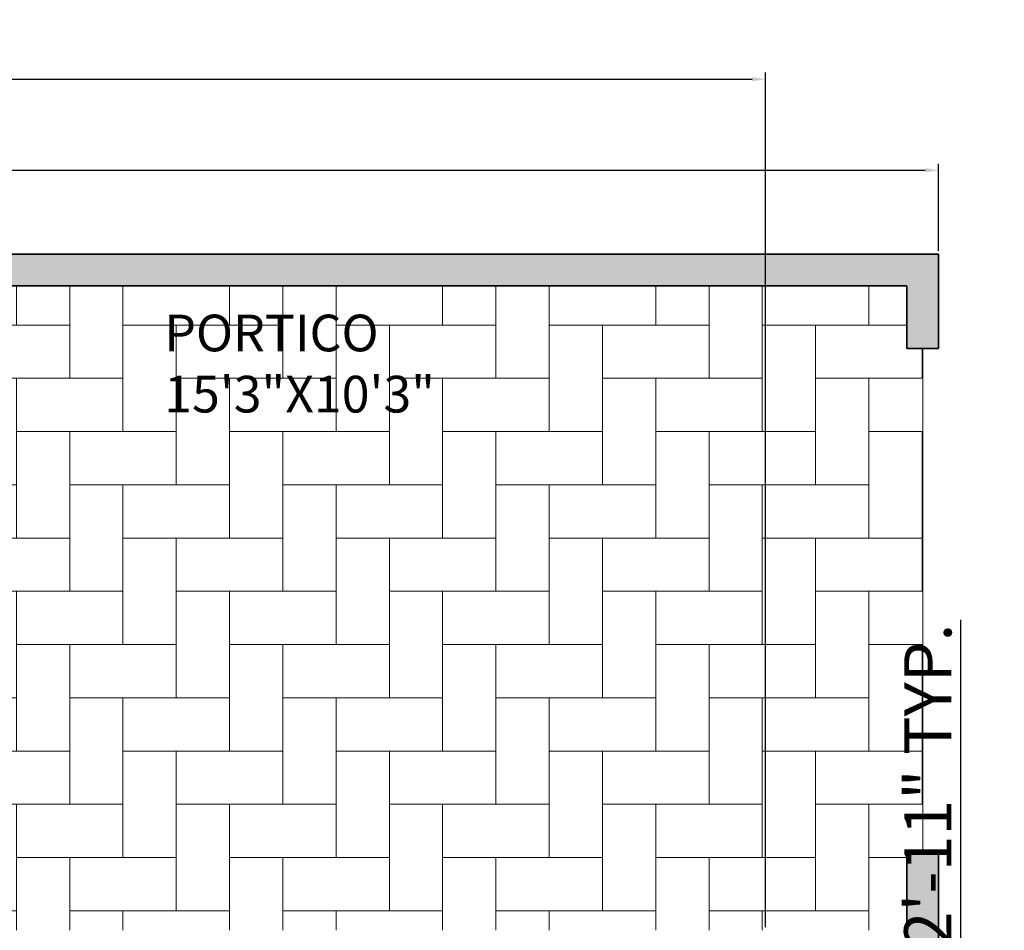
# Model space of a CAD drawing. Units: inches. Extents: x 2337 to 3570, y 1258 to 1938.
# Tile 30 of 30: x 3293 to 3480, y 1764 to 1938. Entities that reach past the tile are written whole.
import ezdxf

# ---------------------------------------------------------------- set-up
doc = ezdxf.new("R2010")
doc.units = ezdxf.units.IN
for name, color, linetype, lineweight in [('A-ANNO-DIMS', 2, 'Continuous', 18), ('A-AREA-IDEN', 7, 'Continuous', 18), ('A-FLOR-PATT', 252, 'Continuous', 13), ('C-PROP', 7, 'Continuous', 35), ('L-SITE-GATE', 4, 'Continuous', 18)]:
    doc.layers.add(name, color=color, linetype=linetype, lineweight=lineweight)
doc.layers.add('C-PROP-PATT', color=251, linetype='Continuous', lineweight=13, true_color=0x636466)
doc.styles.get("Standard").update_dxf_attribs({"font": 'arial.ttf'})
doc.dimstyles.new('ISO-25', dxfattribs={"dimtxt": 9, "dimasz": 2.5, "dimexe": 1.25, "dimexo": 0.625, "dimtad": 1, "dimdec": 1, "dimlunit": 3, "dimtxsty": 'Standard', "dimcen": 2.5, "dimadec": 0, "dimazin": 0, "dimtfac": 1, "dimtdec": 1, "dimtmove": 0, "dimatfit": 3, "dimfxl": 1, "dimarcsym": 0})

# ---------------------------------------------------------------- blocks, each defined once
blk = doc.blocks.new('*D4')
at = {"layer": 'A-ANNO-DIMS', "color": 0, "lineweight": -2, "transparency": 16777216}
for p, q in [((2987.79, 1893.74), (2987.79, 1910.39)), ((3467.79, 1893.74), (3467.79, 1910.39)), ((2990.29, 1909.14), (3465.29, 1909.14))]:
    blk.add_line(p, q, dxfattribs=at)
at = {"layer": 'A-ANNO-DIMS', "color": 0, "transparency": 16777216}
for points in [[(2990.29, 1909.55), (2990.29, 1908.72), (2987.79, 1909.14)], [(3465.29, 1909.55), (3465.29, 1908.72), (3467.79, 1909.14)]]:
    blk.add_solid(points, dxfattribs=at)
at = {"layer": 'Defpoints', "color": 0, "transparency": 16777216}
for p in [(3467.79, 1909.14), (2987.79, 1893.12), (3467.79, 1893.12)]:
    blk.add_point(p, dxfattribs=at)
at = {"layer": 'A-ANNO-DIMS', "color": 0, "transparency": 16777216, "insert": (3227.79, 1914.36), "char_height": 9, "attachment_point": 5}
blk.add_mtext("40'", dxfattribs=at)
blk = doc.blocks.new('*D49')
at = {"layer": 'A-ANNO-DIMS', "color": 0, "lineweight": -2, "transparency": 16777216}
for p, q in [((3472.08, 1757.63), (3472.08, 1823.39)), ((3467.48, 1757.63), (3473.33, 1757.63)), ((3472.08, 1725.34), (3472.08, 1755.13)), ((3467.48, 1722.84), (3473.33, 1722.84))]:
    blk.add_line(p, q, dxfattribs=at)
at = {"layer": 'A-ANNO-DIMS', "color": 0, "transparency": 16777216}
for points in [[(3471.67, 1755.13), (3472.5, 1755.13), (3472.08, 1757.63)], [(3471.67, 1725.34), (3472.5, 1725.34), (3472.08, 1722.84)]]:
    blk.add_solid(points, dxfattribs=at)
at = {"layer": 'Defpoints', "color": 0, "transparency": 16777216}
for p in [(3466.85, 1757.63), (3472.08, 1757.63), (3466.85, 1722.84)]:
    blk.add_point(p, dxfattribs=at)
at = {"layer": 'A-ANNO-DIMS', "color": 0, "transparency": 16777216, "insert": (3466.94, 1791.76), "char_height": 9, "attachment_point": 5, "rotation": 90}
blk.add_mtext('2\'-11" TYP.', dxfattribs=at)
blk = doc.blocks.new('*D111')
at = {"layer": 'A-ANNO-DIMS', "color": 0, "lineweight": -2, "transparency": 16777216}
for p, q in [((3017.79, 1857.74), (3017.79, 1927.77)), ((3020.29, 1926.52), (3432.29, 1926.52)), ((3434.79, 1764.74), (3434.79, 1927.77))]:
    blk.add_line(p, q, dxfattribs=at)
at = {"layer": 'A-ANNO-DIMS', "color": 0, "transparency": 16777216}
for points in [[(3020.29, 1926.93), (3020.29, 1926.1), (3017.79, 1926.52)], [(3432.29, 1926.93), (3432.29, 1926.1), (3434.79, 1926.52)]]:
    blk.add_solid(points, dxfattribs=at)
at = {"layer": 'Defpoints', "color": 0, "transparency": 16777216}
for p in [(3434.79, 1926.52), (3017.79, 1857.12), (3434.79, 1764.12)]:
    blk.add_point(p, dxfattribs=at)
at = {"layer": 'A-ANNO-DIMS', "color": 0, "transparency": 16777216, "insert": (3226.29, 1931.74), "char_height": 9, "attachment_point": 5}
blk.add_mtext('34\'-9"', dxfattribs=at)

msp = doc.modelspace()

# ---------------------------------------------------------------- hatches: boundary and pattern name
at = {"layer": 'A-FLOR-PATT'}
h = msp.add_hatch(dxfattribs=at)
h.set_pattern_fill('AR-HBONE', color=256, scale=0.1, angle=45)
h.set_pattern_definition([(90, (-558.681, 0), (-10.16, 10.16), [30.48, -10.16]), (180, (-558.681, 10.16), (-10.16, 10.16), [30.48, -10.16])])
h.paths.add_polyline_path([(3281.79, 1810.12), (3281.79, 1764.12), (3434.79, 1764.12), (3461.79, 1764.12), (3461.79, 1779.12), (3464.79, 1779.12), (3464.79, 1875.12), (3461.79, 1875.12), (3461.79, 1887.12), (3233.79, 1887.12), (3233.79, 1857.12), (3243.79, 1857.12), (3243.79, 1810.12)])
h.paths.add_polyline_path([(3250.98, 1816.17), (3263.22, 1816.17), (3263.22, 1823.8), (3250.98, 1823.8)], flags=24)
h.paths.add_polyline_path([(3317.33, 1858.95), (3370.67, 1858.95), (3370.67, 1885.07), (3317.33, 1885.07)], flags=24)
at = {"layer": 'C-PROP-PATT'}
h = msp.add_hatch(color=256, dxfattribs=at)
h.dxf.hatch_style = 1
h.paths.add_polyline_path([(3467.79, 1893.12), (2987.79, 1893.12), (2987.79, 1293.12), (3293.79, 1293.12), (3293.79, 1299.12), (2993.79, 1299.12), (2993.79, 1887.12), (3461.79, 1887.12), (3461.79, 1875.12), (3467.79, 1875.12)])
h.paths.add_polyline_path([(3407.79, 1299.12), (3389.79, 1299.12), (3389.79, 1293.12), (3407.79, 1293.12)], flags=17)
h.paths.add_polyline_path([(3461.79, 1299.12), (3455.79, 1299.12), (3455.79, 1293.12), (3467.79, 1293.12), (3467.79, 1779.12), (3461.79, 1779.12)], flags=17)

# ---------------------------------------------------------------- linework, layer by layer
at = {"layer": 'C-PROP'}
for p, q in [((2987.79, 1893.12), (3467.79, 1893.12)), ((3467.79, 1893.12), (3467.79, 1875.12)), ((2993.79, 1887.12), (3461.79, 1887.12)), ((3461.79, 1887.12), (3461.79, 1875.12)), ((3461.79, 1875.12), (3467.79, 1875.12)), ((3461.79, 1779.12), (3461.79, 1299.12)), ((3461.79, 1779.12), (3467.79, 1779.12)), ((3467.79, 1779.12), (3467.79, 1293.12))]:
    msp.add_line(p, q, dxfattribs=at)
at = {"layer": 'L-SITE-GATE'}
msp.add_line((3464.79, 1875.12), (3464.79, 1779.12), dxfattribs=at)

# ---------------------------------------------------------------- texts
at = {"layer": 'A-AREA-IDEN', "insert": (3320.15, 1881.59), "char_height": 7, "attachment_point": 1}
msp.add_mtext_dynamic_manual_height_columns('PORTICO\\P15\'3"X10\'3"', width=66.911, gutter_width=12.5, heights=[0], dxfattribs=at)

# ---------------------------------------------------------------- dimensions: what is measured, and where the dimension line sits
at = {"layer": 'A-ANNO-DIMS'}
for base, p1, p2, override, picture, middle in [((3434.79, 1926.52), (3017.79, 1857.12), (3434.79, 1764.12), {"dimdec": 1, "dimlfac": 1, "dimrnd": 0, "dimzin": 1, "dimdsep": 46, "dimlunit": 4, "dimfrac": 2}, '*D111', (3226.29, 1931.74)), ((3467.79, 1909.14), (2987.79, 1893.12), (3467.79, 1893.12), {"dimclrd": 0, "dimclre": 0, "dimclrt": 0}, '*D4', (3227.79, 1914.36))]:
    dim = msp.add_linear_dim(base=base, p1=p1, p2=p2, dimstyle='ISO-25', override=override, dxfattribs=at)
    dim.commit()
    dim.dimension.update_dxf_attribs({"geometry": picture, "text_midpoint": middle})
dim = msp.add_linear_dim(base=(3472.08, 1757.63), p1=(3466.85, 1722.84), p2=(3466.85, 1757.63), angle=90, text='<> TYP.', dimstyle='ISO-25', override={"dimdec": 1, "dimlfac": 1, "dimrnd": 0, "dimzin": 1, "dimdsep": 46, "dimlunit": 4, "dimfrac": 2}, dxfattribs=at)
dim.commit()
dim.dimension.update_dxf_attribs({"geometry": '*D49', "text_midpoint": (3466.94, 1791.76)})

doc.saveas('drawing.dxf')
